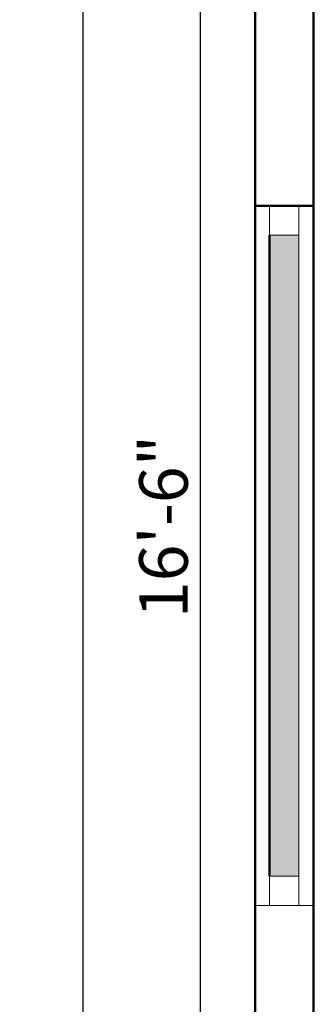
# Model space of a CAD drawing. Units: inches. Extents: x 3064 to 19385, y 846 to 15425.
# Tile 37 of 108: x 5167 to 5197, y 1028 to 1129. Entities that reach past the tile are written whole.
import ezdxf

# ---------------------------------------------------------------- set-up
doc = ezdxf.new("R2010")
doc.units = ezdxf.units.IN
for name, color, linetype, lineweight in [('A-ANNO-DIMS', 2, 'Continuous', 18), ('A-GLAZ', 4, 'Continuous', 18), ('A-WALL', 7, 'Continuous', 50)]:
    doc.layers.add(name, color=color, linetype=linetype, lineweight=lineweight)
doc.styles.get("Standard").update_dxf_attribs({"font": 'arial.ttf'})
doc.dimstyles.new('ISO-25', dxfattribs={"dimtxt": 9, "dimasz": 2.5, "dimexe": 1.25, "dimexo": 0.625, "dimtad": 1, "dimdec": 1, "dimlunit": 3, "dimtxsty": 'Standard', "dimcen": 2.5, "dimadec": 0, "dimazin": 0, "dimtfac": 1, "dimtdec": 1, "dimtmove": 0, "dimatfit": 3, "dimfxl": 1, "dimarcsym": 0})

# ---------------------------------------------------------------- blocks, each defined once
blk = doc.blocks.new('*D70')
at = {"layer": 'A-ANNO-DIMS', "color": 0, "lineweight": -2, "transparency": 16777216}
for p, q in [((5196.39, 1176.1), (5184.17, 1176.1)), ((5185.42, 980.6), (5185.42, 1173.6)), ((5196.39, 978.1), (5184.17, 978.1))]:
    blk.add_line(p, q, dxfattribs=at)
at = {"layer": 'A-ANNO-DIMS', "color": 0, "transparency": 16777216}
for points in [[(5185, 1173.6), (5185.83, 1173.6), (5185.42, 1176.1)], [(5185, 980.6), (5185.83, 980.6), (5185.42, 978.1)]]:
    blk.add_solid(points, dxfattribs=at)
at = {"layer": 'Defpoints', "color": 0, "transparency": 16777216}
for p in [(5185.42, 1176.1), (5197.02, 1176.1), (5197.02, 978.1)]:
    blk.add_point(p, dxfattribs=at)
at = {"layer": 'A-ANNO-DIMS', "color": 0, "transparency": 16777216, "insert": (5182.24, 1077.1), "char_height": 5, "attachment_point": 5, "rotation": 90}
blk.add_mtext('16\'-6"', dxfattribs=at)
blk = doc.blocks.new('*D76')
at = {"layer": 'A-ANNO-DIMS', "color": 0, "lineweight": -2, "transparency": 16777216}
for p, q in [((5190.39, 1392.1), (5172.09, 1392.1)), ((5173.34, 902.6), (5173.34, 1389.6)), ((5190.39, 900.1), (5172.09, 900.1))]:
    blk.add_line(p, q, dxfattribs=at)
at = {"layer": 'A-ANNO-DIMS', "color": 0, "transparency": 16777216}
for points in [[(5172.92, 1389.6), (5173.75, 1389.6), (5173.34, 1392.1)], [(5172.92, 902.6), (5173.75, 902.6), (5173.34, 900.1)]]:
    blk.add_solid(points, dxfattribs=at)
at = {"layer": 'Defpoints', "color": 0, "transparency": 16777216}
for p in [(5173.34, 1392.1), (5191.02, 1392.1), (5191.02, 900.1)]:
    blk.add_point(p, dxfattribs=at)
at = {"layer": 'A-ANNO-DIMS', "color": 0, "transparency": 16777216, "insert": (5170.2, 1146.1), "char_height": 5, "attachment_point": 5, "rotation": 90}
blk.add_mtext("41'", dxfattribs=at)
blk = doc.blocks.new('WIN-1900')
blk.add_line((3, 0), (3, 66))
blk.add_lwpolyline([(3, 66), (0, 66), (0, 69), (3, 69)], close=True)

msp = doc.modelspace()

# ---------------------------------------------------------------- hatches: boundary and pattern name
at = {"layer": 'A-GLAZ'}
h = msp.add_hatch(color=256, dxfattribs=at)
h.dxf.hatch_style = 1
h.paths.add_polyline_path([(5192.52, 1041.1), (5195.52, 1041.1), (5195.52, 1107.1), (5192.52, 1107.1)])

# ---------------------------------------------------------------- linework, layer by layer
msp.add_line((5197.02, 1038.1), (5191.02, 1038.1), dxfattribs=at)
msp.add_lwpolyline([(5195.52, 1038.1), (5192.52, 1038.1), (5192.52, 1041.1), (5195.52, 1041.1)], close=True, dxfattribs=at)
at = {"layer": 'A-WALL'}
for p, q in [((5191.02, 1392.1), (5191.02, 972.1)), ((5197.02, 1176.1), (5197.02, 978.1)), ((5197.02, 1110.1), (5191.02, 1110.1)), ((5192.52, 1041.1), (5192.52, 1107.1))]:
    msp.add_line(p, q, dxfattribs=at)

# ---------------------------------------------------------------- block references
at = {"layer": 'A-GLAZ'}
msp.add_blockref('WIN-1900', (5192.52, 1041.1), dxfattribs=at)

# ---------------------------------------------------------------- dimensions: what is measured, and where the dimension line sits
at = {"layer": 'A-ANNO-DIMS'}
for base, p1, p2, override, picture, middle in [((5173.34, 1392.1), (5191.02, 900.1), (5191.02, 1392.1), {"dimtxt": 5, "dimclrd": 0, "dimclre": 0, "dimclrt": 0}, '*D76', (5170.2, 1146.1)), ((5185.42, 1176.1), (5197.02, 978.1), (5197.02, 1176.1), {"dimtxt": 5, "dimclrd": 0, "dimclre": 0, "dimclrt": 0, "dimtmove": 1}, '*D70', (5182.24, 1077.1))]:
    dim = msp.add_linear_dim(base=base, p1=p1, p2=p2, angle=90, dimstyle='ISO-25', override=override, dxfattribs=at)
    dim.commit()
    dim.dimension.update_dxf_attribs({"geometry": picture, "text_midpoint": middle})

doc.saveas('drawing.dxf')
